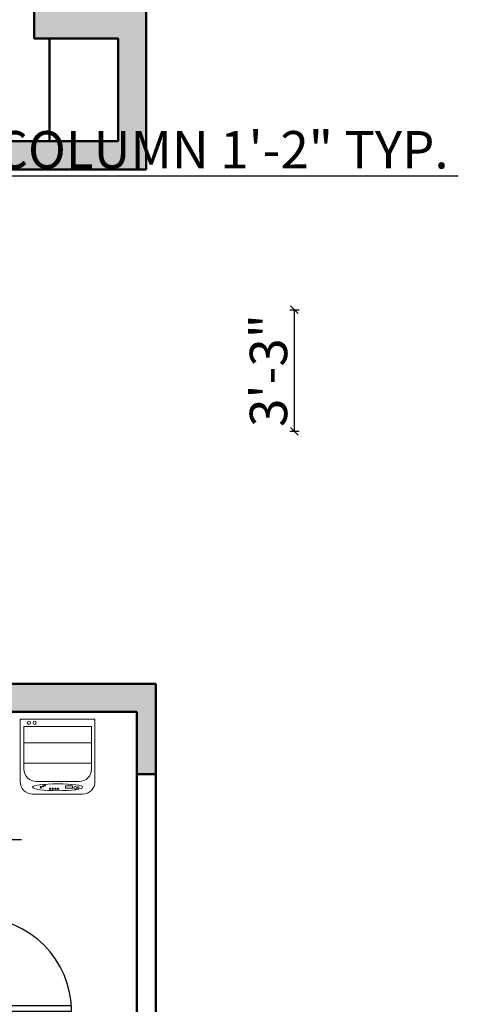
# Model space of a CAD drawing. Units: inches. Extents: x 375 to 1122, y 27 to 1069.
# Tile 82 of 155: x 945 to 1086, y 400 to 716. Entities that reach past the tile are written whole.
import ezdxf

# ---------------------------------------------------------------- set-up
doc = ezdxf.new("R2010")
doc.units = ezdxf.units.IN
for name, color, linetype, lineweight in [('A-ANNO-DIMS', 2, 'Continuous', 18), ('A-EQPM', 55, 'Continuous', 18), ('A-WALL-PATT', 252, 'Continuous', 13), ('Doors', 150, 'Continuous', 25), ('Walls', 250, 'Continuous', 50)]:
    doc.layers.add(name, color=color, linetype=linetype, lineweight=lineweight)
doc.styles.get("Standard").update_dxf_attribs({"font": 'arial.ttf'})
doc.dimstyles.new('ISO-25', dxfattribs={"dimtxt": 12, "dimasz": 2.5, "dimexe": 1.5, "dimexo": 1.5, "dimtad": 1, "dimdec": 1, "dimlunit": 3, "dimtxsty": 'Standard', "dimblk": 'ARCHTICK', "dimcen": 2.5, "dimadec": 0, "dimazin": 0, "dimtfac": 1, "dimtdec": 1, "dimtmove": 0, "dimatfit": 3, "dimfxl": 1.5, "dimfxlon": 1, "dimarcsym": 0})

# ---------------------------------------------------------------- blocks, each defined once
blk = doc.blocks.new('*U13')
for p, q in [((-30, 0), (-30, -4)), ((0, 0), (0, -4))]:
    blk.add_line(p, q)
blk.add_lwpolyline([(0, 0), (0, 30), (-1.75, 30), (-1.75, 0)], close=True)
blk.add_arc((0, 0), 30, 90, 180)
blk = doc.blocks.new('A$C20C229D7')
for p, q in [((0, 600), (0, 580)), ((24, 600), (0, 600)), ((24, 580), (24, 600)), ((22.88, 597.68), (1.21, 597.68)), ((1.21, 597.68), (1.21, 584)), ((22.88, 584), (22.88, 597.68)), ((1.21, 592.39), (22.88, 592.39)), ((1.21, 585.92), (22.88, 585.92)), ((5.21, 580), (18.88, 580)), ((14.51, 578.61), (16.76, 578.61)), ((14.51, 577.92), (14.51, 578.61)), ((16.76, 577.92), (14.51, 577.92)), ((16.76, 578.61), (16.76, 577.92)), ((4, 576), (20, 576))]:
    blk.add_line(p, q)
for centre, radius in [((2.81, 598.86), 0.52), ((4.66, 598.86), 0.52), ((6.67, 578.16), 0.267), ((7.36, 578.48), 0.187), ((7.95, 578.72), 0.133), ((9.61, 577.68), 0.24), ((10.46, 577.68), 0.24), ((11.31, 577.68), 0.24), ((12.11, 577.68), 0.24), ((17.64, 578), 0.4), ((18.62, 578.05), 0.293)]:
    blk.add_circle(centre, radius)
for centre, start, end in [((5.21, 584), 180, 270), ((18.88, 584), 270, 0), ((4, 580), 180, 270), ((20, 580), 270, 0)]:
    blk.add_arc(centre, 4, start, end)
blk.add_ellipse((12.07, 578.17), major_axis=(8.08, 0), ratio=0.137115)
blk = doc.blocks.new('_ArchTick')
at = {"color": 0, "linetype": 'ByBlock', "const_width": 0.15}
blk.add_lwpolyline([(-0.5, -0.5), (0.5, 0.5)], dxfattribs=at)
blk = doc.blocks.new('*D41')
at = {"layer": 'A-ANNO-DIMS', "color": 0, "lineweight": -2, "transparency": 16777216}
for p, q in [((918.01, 666.03), (918.01, 663.93)), ((918.01, 665.43), (932.01, 665.43)), ((932.01, 666.03), (932.01, 663.93)), ((932.01, 665.43), (1086.07, 665.43))]:
    blk.add_line(p, q, dxfattribs=at)
at = {"layer": 'Defpoints', "color": 0, "transparency": 16777216}
for p in [(918.01, 667.53), (932.01, 667.53), (932.01, 665.43)]:
    blk.add_point(p, dxfattribs=at)
at = {"layer": 'A-ANNO-DIMS', "color": 0, "lineweight": -2, "transparency": 16777216, "xscale": 2.5, "yscale": 2.5, "zscale": 2.5, "rotation": 180}
blk.add_blockref('_ArchTick', (918.01, 665.43), dxfattribs=at)
at = {"layer": 'A-ANNO-DIMS', "color": 0, "lineweight": -2, "transparency": 16777216, "xscale": 2.5, "yscale": 2.5, "zscale": 2.5}
blk.add_blockref('_ArchTick', (932.01, 665.43), dxfattribs=at)
at = {"layer": 'A-ANNO-DIMS', "color": 0, "transparency": 16777216, "insert": (1010.29, 672.26), "char_height": 12, "attachment_point": 5}
blk.add_mtext('COLUMN 1\'-2" TYP.', dxfattribs=at)
blk = doc.blocks.new('*D53')
at = {"layer": 'A-ANNO-DIMS', "color": 0, "lineweight": -2, "transparency": 16777216}
for p, q in [((669.51, 454.15), (669.51, 451.15)), ((669.51, 452.65), (722.01, 452.65)), ((722.01, 454.15), (722.01, 451.15)), ((722.01, 452.65), (946.03, 452.65))]:
    blk.add_line(p, q, dxfattribs=at)
at = {"layer": 'Defpoints', "color": 0, "transparency": 16777216}
for p in [(669.51, 460.53), (722.01, 460.53), (722.01, 452.65)]:
    blk.add_point(p, dxfattribs=at)
at = {"layer": 'A-ANNO-DIMS', "color": 0, "lineweight": -2, "transparency": 16777216, "xscale": 2.5, "yscale": 2.5, "zscale": 2.5, "rotation": 180}
blk.add_blockref('_ArchTick', (669.51, 452.65), dxfattribs=at)
at = {"layer": 'A-ANNO-DIMS', "color": 0, "lineweight": -2, "transparency": 16777216, "xscale": 2.5, "yscale": 2.5, "zscale": 2.5}
blk.add_blockref('_ArchTick', (722.01, 452.65), dxfattribs=at)
at = {"layer": 'A-ANNO-DIMS', "color": 0, "transparency": 16777216, "insert": (835.27, 459.49), "char_height": 12, "attachment_point": 5}
blk.add_mtext('SHOWER PAN 4\'-4 1/2" TYP.', dxfattribs=at)
blk = doc.blocks.new('*D84')
at = {"layer": 'A-ANNO-DIMS', "color": 0, "lineweight": -2, "transparency": 16777216}
for p, q in [((845.01, 117.53), (845.01, 114.53)), ((950.01, 117.53), (950.01, 114.53)), ((845.01, 116.03), (950.01, 116.03))]:
    blk.add_line(p, q, dxfattribs=at)
at = {"layer": 'Defpoints', "color": 0, "transparency": 16777216}
for p in [(845.01, 814.53), (950.01, 814.53), (950.01, 116.03)]:
    blk.add_point(p, dxfattribs=at)
at = {"layer": 'A-ANNO-DIMS', "color": 0, "lineweight": -2, "transparency": 16777216, "xscale": 2.5, "yscale": 2.5, "zscale": 2.5, "rotation": 180}
blk.add_blockref('_ArchTick', (845.01, 116.03), dxfattribs=at)
at = {"layer": 'A-ANNO-DIMS', "color": 0, "lineweight": -2, "transparency": 16777216, "xscale": 2.5, "yscale": 2.5, "zscale": 2.5}
blk.add_blockref('_ArchTick', (950.01, 116.03), dxfattribs=at)
at = {"layer": 'A-ANNO-DIMS', "color": 0, "transparency": 16777216, "insert": (897.51, 122.78), "char_height": 12, "attachment_point": 5}
blk.add_mtext('8\'-9"', dxfattribs=at)
blk = doc.blocks.new('*D86')
at = {"layer": 'A-ANNO-DIMS', "color": 0, "lineweight": -2, "transparency": 16777216}
for p, q in [((1032.01, 622.53), (1035.01, 622.53)), ((1033.51, 583.53), (1033.51, 622.53)), ((1032.01, 583.53), (1035.01, 583.53))]:
    blk.add_line(p, q, dxfattribs=at)
at = {"layer": 'Defpoints', "color": 0, "transparency": 16777216}
for p in [(884.01, 622.53), (1033.51, 622.53), (884.01, 583.53)]:
    blk.add_point(p, dxfattribs=at)
at = {"layer": 'A-ANNO-DIMS', "color": 0, "lineweight": -2, "transparency": 16777216, "xscale": 2.5, "yscale": 2.5, "zscale": 2.5}
for p, rotation in [((1033.51, 622.53), 90), ((1033.51, 583.53), 270)]:
    blk.add_blockref('_ArchTick', p, dxfattribs=dict(at, rotation=rotation))
at = {"layer": 'A-ANNO-DIMS', "color": 0, "transparency": 16777216, "insert": (1026.75, 603.03), "char_height": 12, "attachment_point": 5, "rotation": 90}
blk.add_mtext('3\'-3"', dxfattribs=at)

msp = doc.modelspace()

# ---------------------------------------------------------------- hatches: boundary and pattern name
at = {"layer": 'A-WALL-PATT'}
h = msp.add_hatch(color=256, dxfattribs=at)
h.dxf.hatch_style = 1
h.paths.add_polyline_path([(962.01, 388.53), (989.01, 388.53), (989.01, 394.53), (962.01, 394.53), (932.01, 394.53), (932.01, 397.53), (923.01, 397.53), (923.01, 394.53), (842.01, 394.53), (842.01, 334.53), (839.51, 334.53), (839.51, 328.53), (854.01, 328.53), (854.01, 334.53), (848.01, 334.53), (848.01, 388.53), (953.01, 388.53), (953.01, 356.08), (962.01, 356.08), (962.01, 358.55), (989.01, 358.55), (989.01, 364.55), (962.01, 364.55)])
h.paths.add_polyline_path([(989.01, 502.53), (932.01, 502.53), (932.01, 583.53), (932.01, 593.53), (923.01, 593.53), (923.01, 583.53), (854.01, 583.53), (854.01, 556.53), (863.01, 556.53), (863.01, 574.53), (923.01, 574.53), (923.01, 502.53), (863.01, 502.53), (863.01, 520.53), (854.01, 520.53), (854.01, 502.53), (773.01, 502.53), (773.01, 493.53), (788.01, 493.53), (788.01, 402.03), (722.01, 402.03), (722.01, 373.53), (728.01, 373.53), (728.01, 396.03), (788.01, 396.03), (788.01, 373.53), (794.01, 373.53), (794.01, 430.53), (814.01, 430.53), (814.01, 436.53), (794.01, 436.53), (794.01, 493.53), (923.01, 493.53), (923.01, 487.53), (932.01, 487.53), (932.01, 493.53), (983.01, 493.53), (983.01, 473.53), (989.01, 473.53)])
h.paths.add_polyline_path([(797.01, 325.53), (805.01, 325.53), (805.01, 328.53), (807.51, 328.53), (807.51, 334.53), (791.01, 334.53), (791.01, 226.53), (770.76, 226.53), (770.76, 217.53), (791.01, 217.53), (791.01, 187.53), (855.01, 187.53), (855.01, 196.53), (797.01, 196.53)])
h.paths.add_polyline_path([(989.01, 238.53), (962.01, 238.53), (962.01, 256.42), (953.01, 256.42), (953.01, 229.53), (980.01, 229.53), (980.01, 196.53), (915.01, 196.53), (915.01, 187.53), (989.01, 187.53)])
h.paths.add_polyline_path([(962.01, 334.53), (884.01, 334.53), (884.01, 328.53), (918.01, 328.53), (918.01, 325.53), (932.01, 325.53), (932.01, 328.53), (953.01, 328.53), (953.01, 304.42), (962.01, 304.42)])
h.paths.add_polyline_path([(606.51, 283.53), (609.51, 283.53), (609.51, 289.53), (600.51, 289.53), (600.51, 196.53), (578.51, 196.53), (578.51, 187.53), (606.51, 187.53), (606.51, 196.53)])
h.paths.add_polyline_path([(666.51, 292.53), (660.51, 292.53), (660.51, 289.53), (633.51, 289.53), (633.51, 283.53), (660.51, 283.53), (660.51, 196.53), (628.01, 196.53), (628.01, 187.53), (630.53, 187.53), (630.53, 160.53), (636.53, 160.53), (636.53, 187.53), (660.51, 187.53), (660.51, 160.53), (666.51, 160.53), (666.51, 217.53), (686.76, 217.53), (686.76, 226.53), (666.51, 226.53)])
h.paths.add_polyline_path([(480.51, 256.42), (471.51, 256.42), (471.51, 238.53), (444.51, 238.53), (444.51, 187.53), (518.51, 187.53), (518.51, 196.53), (453.51, 196.53), (453.51, 229.53), (480.51, 229.53)])
h.paths.add_polyline_path([(480.51, 328.53), (652.51, 328.53), (652.51, 325.53), (660.51, 325.53), (660.51, 322.53), (666.51, 322.53), (666.51, 334.53), (507.51, 334.53), (507.51, 360.53), (498.51, 360.53), (498.51, 334.53), (471.51, 334.53), (471.51, 304.42), (480.51, 304.42)])
h.paths.add_polyline_path([(507.51, 484.53), (498.51, 484.53), (498.51, 444.53), (507.51, 444.53), (507.51, 454.53), (621.51, 454.53), (621.51, 460.53), (507.51, 460.53)])
h.paths.add_polyline_path([(672.51, 604.53), (683.26, 604.53), (683.26, 613.53), (669.51, 613.53), (669.51, 649.53), (663.51, 649.53), (663.51, 589.53), (507.51, 589.53), (507.51, 613.53), (498.51, 613.53), (498.51, 556.53), (507.51, 556.53), (507.51, 580.53), (663.51, 580.53), (663.51, 520.53), (669.51, 520.53), (669.51, 556.53), (683.26, 556.53), (683.26, 565.53), (672.51, 565.53)])
h.paths.add_polyline_path([(731.01, 667.53), (734.01, 667.53), (734.01, 676.53), (728.01, 676.53), (728.01, 715.53), (657.51, 715.53), (657.51, 709.53), (663.51, 709.53), (663.51, 673.53), (669.51, 673.53), (669.51, 709.53), (722.01, 709.53), (722.01, 613.53), (704.76, 613.53), (704.76, 604.53), (722.01, 604.53), (722.01, 565.53), (704.76, 565.53), (704.76, 556.53), (722.01, 556.53), (722.01, 502.53), (722.01, 460.53), (669.51, 460.53), (669.51, 496.53), (663.51, 496.53), (663.51, 460.53), (657.51, 460.53), (657.51, 454.53), (728.01, 454.53), (728.01, 493.53), (734.01, 493.53), (734.01, 502.53), (731.01, 502.53)])
h.paths.add_polyline_path([(986.01, 718.53), (959.01, 718.53), (959.01, 727.53), (950.01, 727.53), (950.01, 709.53), (977.01, 709.53), (977.01, 676.53), (794.01, 676.53), (794.01, 805.53), (802.01, 805.53), (802.01, 808.53), (804.51, 808.53), (804.51, 814.53), (788.01, 814.53), (788.01, 774.03), (728.01, 774.03), (728.01, 796.53), (722.01, 796.53), (722.01, 768.03), (788.01, 768.03), (788.01, 676.53), (773.01, 676.53), (773.01, 667.53), (923.01, 667.53), (923.01, 657.53), (932.01, 657.53), (932.01, 667.53), (986.01, 667.53)])
h.paths.add_polyline_path([(621.51, 715.53), (507.51, 715.53), (507.51, 733.53), (498.51, 733.53), (498.51, 715.53), (498.51, 685.53), (507.51, 685.53), (507.51, 709.53), (621.51, 709.53)])
h.paths.add_polyline_path([(666.51, 847.03), (660.51, 847.03), (660.51, 844.53), (652.51, 844.53), (652.51, 841.53), (480.51, 841.53), (480.51, 859.53), (471.51, 859.53), (471.51, 835.53), (498.51, 835.53), (498.51, 817.53), (507.51, 817.53), (507.51, 835.53), (666.51, 835.53)])
h.paths.add_polyline_path([(480.51, 940.53), (453.51, 940.53), (453.51, 973.53), (518.51, 973.53), (518.51, 982.53), (444.51, 982.53), (444.51, 931.53), (471.51, 931.53), (471.51, 907.53), (480.51, 907.53)])
h.paths.add_polyline_path([(606.51, 982.53), (578.51, 982.53), (578.51, 973.53), (600.51, 973.53), (600.51, 880.53), (609.51, 880.53), (609.51, 886.53), (606.51, 886.53)])
h.paths.add_polyline_path([(666.51, 943.53), (686.76, 943.53), (686.76, 952.53), (666.51, 952.53), (666.51, 1009.53), (660.51, 1009.53), (660.51, 982.53), (636.53, 982.53), (636.53, 1009.53), (630.53, 1009.53), (630.53, 982.53), (628.01, 982.53), (628.01, 973.53), (660.51, 973.53), (660.51, 886.53), (633.51, 886.53), (633.51, 880.53), (660.51, 880.53), (660.51, 877.03), (666.51, 877.03)])
h.paths.add_polyline_path([(986.01, 874.53), (932.01, 874.53), (932.01, 877.53), (923.01, 877.53), (923.01, 874.53), (788.01, 874.53), (788.01, 868.53), (788.01, 844.53), (794.01, 844.53), (794.01, 868.53), (839.01, 868.53), (839.01, 814.53), (836.51, 814.53), (836.51, 808.53), (851.01, 808.53), (851.01, 814.53), (845.01, 814.53), (845.01, 868.53), (986.01, 868.53)])
h.paths.add_polyline_path([(959.01, 838.55), (986.01, 838.55), (986.01, 844.55), (959.01, 844.55), (959.01, 847.03), (950.01, 847.03), (950.01, 814.53), (881.01, 814.53), (881.01, 808.53), (918.01, 808.53), (918.01, 805.53), (932.01, 805.53), (932.01, 808.53), (950.01, 808.53), (950.01, 793.53), (959.01, 793.53)])
h.paths.add_polyline_path([(986.01, 982.53), (899.01, 982.53), (899.01, 973.53), (923.01, 973.53), (923.01, 967.53), (932.01, 967.53), (932.01, 973.53), (980.01, 973.53), (980.01, 953.53), (986.01, 953.53)])
h.paths.add_polyline_path([(851.01, 982.53), (788.01, 982.53), (788.01, 952.53), (770.76, 952.53), (770.76, 943.53), (788.01, 943.53), (788.01, 910.53), (814.01, 910.53), (814.01, 916.53), (794.01, 916.53), (794.01, 973.53), (851.01, 973.53)])

# ---------------------------------------------------------------- linework, layer by layer
at = {"layer": 'Walls'}
for p, q in [((950.01, 727.53), (950.01, 709.53)), ((986.01, 667.53), (986.01, 718.53)), ((977.01, 709.53), (950.01, 709.53)), ((955.01, 676.53), (955.01, 709.53)), ((977.01, 676.53), (977.01, 709.53)), ((977.01, 676.53), (794.01, 676.53)), ((986.01, 667.53), (932.01, 667.53)), ((989.01, 502.53), (932.01, 502.53)), ((989.01, 394.53), (989.01, 502.53)), ((983.01, 493.53), (932.01, 493.53)), ((983.01, 394.53), (983.01, 493.53)), ((983.01, 473.53), (989.01, 473.53))]:
    msp.add_line(p, q, dxfattribs=at)

# ---------------------------------------------------------------- block references
at = {"layer": 'A-EQPM'}
msp.add_blockref('A$C20C229D7', (945.55, -108.79), dxfattribs=at)
at = {"layer": 'Doors', "rotation": 270}
msp.add_blockref('*U13', (932.01, 397.53), dxfattribs=at)

# ---------------------------------------------------------------- dimensions: what is measured, and where the dimension line sits
at = {"layer": 'A-ANNO-DIMS'}
dim = msp.add_linear_dim(base=(950.01, 116.03), p1=(845.01, 814.53), p2=(950.01, 814.53), dimstyle='ISO-25', override={"dimdec": 1, "dimlfac": 1, "dimrnd": 0, "dimzin": 1, "dimdsep": 46, "dimlunit": 4, "dimfrac": 2}, dxfattribs=at)
dim.commit()
dim.dimension.update_dxf_attribs({"geometry": '*D84', "text_midpoint": (897.51, 122.78)})
for base, p1, p2, text, picture, middle in [((932.01, 665.43), (918.01, 667.53), (932.01, 667.53), 'COLUMN <> TYP.', '*D41', (1010.29, 672.26)), ((722.01, 452.65), (669.51, 460.53), (722.01, 460.53), 'SHOWER PAN <> TYP.', '*D53', (835.27, 459.49))]:
    dim = msp.add_linear_dim(base=base, p1=p1, p2=p2, text=text, dimstyle='ISO-25', override={"dimdec": 1, "dimlfac": 1, "dimrnd": 0, "dimzin": 1, "dimdsep": 46, "dimlunit": 4, "dimfrac": 2}, dxfattribs=at)
    dim.commit()
    dim.dimension.update_dxf_attribs({"geometry": picture, "text_midpoint": middle})
dim = msp.add_linear_dim(base=(1033.51, 622.53), p1=(884.01, 583.53), p2=(884.01, 622.53), angle=90, dimstyle='ISO-25', override={"dimdec": 1, "dimlfac": 1, "dimrnd": 0, "dimzin": 1, "dimdsep": 46, "dimlunit": 4, "dimfrac": 2}, dxfattribs=at)
dim.commit()
dim.dimension.update_dxf_attribs({"geometry": '*D86', "text_midpoint": (1026.75, 603.03)})

doc.saveas('drawing.dxf')
